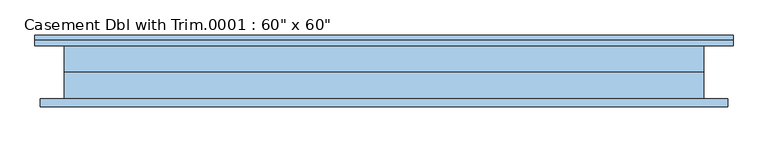
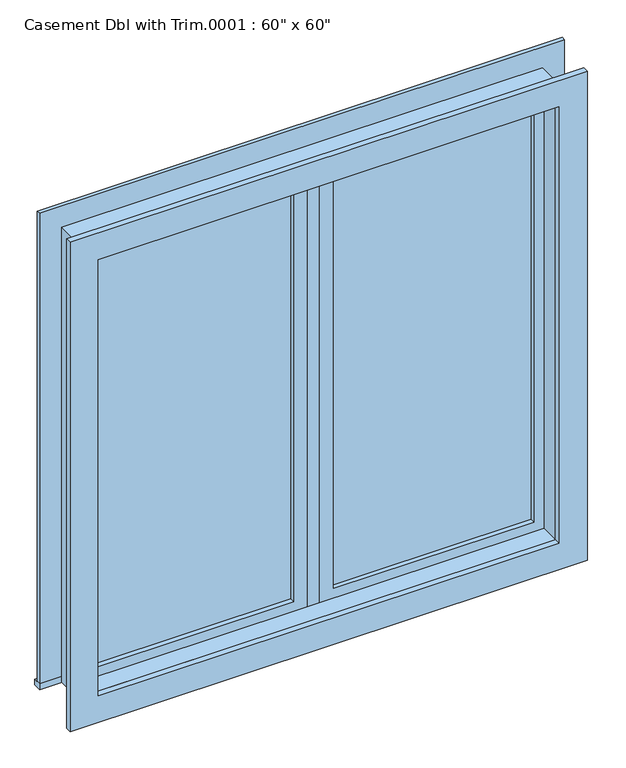
"""IFC4 building model written with IfcOpenShell, lengths in millimetres: window geometry."""

from ifc_helpers import new_model, si_unit, frame, origin, place, context, project, spatial, polyline, outline, extrude, source, transform, mapped, element, save


def window_26183f51(model_context):
    return source(origin(), model_context, "Body", "SweptSolid", [
        extrude(outline(polyline([(63.5, 47.625), (698.5, 47.625), (698.5, 34.925), (63.5, 34.925), (63.5, 47.625)])), frame((0.0, 0.0, 977.9), z_axis=(0.0, 0.0, 1.0), x_axis=(1.0, 0.0, 0.0)), (0.0, 0.0, 1.0), 1397.0),
        extrude(outline(polyline([(2419.35, 19.05), (933.45, 19.05), (933.45, 742.95), (2419.35, 742.95), (2419.35, 19.05)]), holes=[polyline([(2374.9, 63.5), (2374.9, 698.5), (977.9, 698.5), (977.9, 63.5), (2374.9, 63.5)])]), frame((0.0, 19.05, 0.0), z_axis=(0.0, 1.0, 0.0), x_axis=(0.0, 0.0, 1.0)), (0.0, 0.0, 1.0), 44.45),
        extrude(outline(polyline([(19.05, 19.05), (-19.05, 19.05), (-19.05, 82.55), (19.05, 82.55), (19.05, 19.05)])), frame((0.0, 0.0, 933.45), z_axis=(0.0, 0.0, 1.0), x_axis=(1.0, 0.0, 0.0)), (0.0, 0.0, 1.0), 1485.9),
        extrude(outline(polyline([(-831.85, 107.95), (831.85, 107.95), (831.85, 82.55), (-831.85, 82.55), (-831.85, 107.95)])), frame((0.0, 0.0, 914.4), z_axis=(0.0, 0.0, 1.0), x_axis=(1.0, 0.0, 0.0)), (0.0, 0.0, 1.0), 19.05),
        extrude(outline(polyline([(2419.35, -742.95), (2419.35, 742.95), (933.45, 742.95), (933.45, 831.85), (2508.25, 831.85), (2508.25, -831.85), (933.45, -831.85), (933.45, -742.95), (2419.35, -742.95)])), frame((0.0, 82.55, 0.0), z_axis=(0.0, 1.0, 0.0), x_axis=(0.0, 0.0, 1.0)), (0.0, 0.0, 1.0), 12.7),
        extrude(outline(polyline([(2495.55, 819.15), (2495.55, -819.15), (857.25, -819.15), (857.25, 819.15), (2495.55, 819.15)]), holes=[polyline([(2406.65, 730.25), (946.15, 730.25), (946.15, -730.25), (2406.65, -730.25), (2406.65, 730.25)])]), frame((0.0, -63.5, 0.0), z_axis=(0.0, 1.0, 0.0), x_axis=(0.0, 0.0, 1.0)), (0.0, 0.0, 1.0), 19.05),
        extrude(outline(polyline([(-63.5, 34.925), (-698.5, 34.925), (-698.5, 47.625), (-63.5, 47.625), (-63.5, 34.925)])), frame((0.0, 0.0, 977.9), z_axis=(0.0, 0.0, 1.0), x_axis=(1.0, 0.0, 0.0)), (0.0, 0.0, 1.0), 1397.0),
        extrude(outline(polyline([(2419.35, -742.95), (933.45, -742.95), (933.45, -19.05), (2419.35, -19.05), (2419.35, -742.95)]), holes=[polyline([(2374.9, -698.5), (2374.9, -63.5), (977.9, -63.5), (977.9, -698.5), (2374.9, -698.5)])]), frame((0.0, 19.05, 0.0), z_axis=(0.0, 1.0, 0.0), x_axis=(0.0, 0.0, 1.0)), (0.0, 0.0, 1.0), 44.45),
        extrude(outline(polyline([(2438.4, -762.0), (914.4, -762.0), (914.4, 762.0), (2438.4, 762.0), (2438.4, -762.0)]), holes=[polyline([(2406.65, -730.25), (2406.65, 730.25), (946.15, 730.25), (946.15, -730.25), (2406.65, -730.25)])]), frame((0.0, -44.45, 0.0), z_axis=(0.0, 1.0, 0.0), x_axis=(0.0, 0.0, 1.0)), (0.0, 0.0, 1.0), 63.5),
        extrude(outline(polyline([(2438.4, 762.0), (2438.4, -762.0), (914.4, -762.0), (914.4, 762.0), (2438.4, 762.0)]), holes=[polyline([(2419.35, 742.95), (933.45, 742.95), (933.45, -742.95), (2419.35, -742.95), (2419.35, 742.95)])]), frame((0.0, 19.05, 0.0), z_axis=(0.0, 1.0, 0.0), x_axis=(0.0, 0.0, 1.0)), (0.0, 0.0, 1.0), 63.5),
    ])


if __name__ == "__main__":
    model = new_model("IFC4")
    model_context = context("Model", 3, world=origin())
    ifc_project = project(units=[si_unit("LENGTHUNIT", "METRE", prefix="MILLI")], contexts=[model_context])
    site = spatial("IfcSite", under=ifc_project)
    building = spatial("IfcBuilding", under=site)
    placement = place(None, origin())
    window_shape = window_26183f51(model_context)
    element("IfcWindow", 1, ObjectType="Casement Dbl with Trim.0001 : 60\" x 60\"", at=placement, inside=building, context=model_context, shape_type="MappedRepresentation", body=[
        mapped(window_shape, transform((0.0, 0.0, 0.0), x_axis=(1.0, 0.0, 0.0), y_axis=(0.0, 1.0, 0.0), z_axis=(0.0, 0.0, 1.0))),
    ])
    save(model, "model.ifc")

# Revit data of these elements
# Type "Casement Dbl with Trim.0001 : 60\" x 60\""
#   Type Mark = "16"
#   Construction Type Id = "GSP4R"
#   Assembly Code = "B2020100"
#   Analytic Construction = "1/8 in Pilkington single glazing"
#   Visual Light Transmittance = 0.9
#   Solar Heat Gain Coefficient = 0.78
#   Heat Transfer Coefficient (U) = 0.6496 BTU/(h·ft²·°F)
#   Height = 5' - 0"
#   Default Sill Height = 3' - 0"
#   Trim Projection - Ext. = 0' - 0 1/2"
#   Trim Projection - Int. = 0' - 0 3/4"
#   Trim Width - Exterior = 0' - 3 1/2"
#   Trim Width - Interior = 0' - 3 1/2"
#   Width = 5' - 0"
#   Window Inset = 0' - 0 3/4"
#   Define Thermal Properties by = 1
#   Glass Pane Material = Glass
#   Sash Material = Sash
#   Trim Exterior Material = Trim
#   Trim Interior Material = Trim
#   Wall Closure = (empty or 0)
# Element 1 (IfcWindow, "Casement Dbl with Trim.0001 : 60\" x 60\"")
#   Materials on its faces: "Sash", "Trim", "Glass"
# Materials
#   "Glass": class "Glass", colour RGB 0 128 192, transparency 0.75, Description = "Soda Lime Glass", Cost = 0
#   "Sash": class "Wood", colour RGB 224 178 126, transparency 0
#   "Trim": class "Wood", colour RGB 224 178 126, transparency 0
